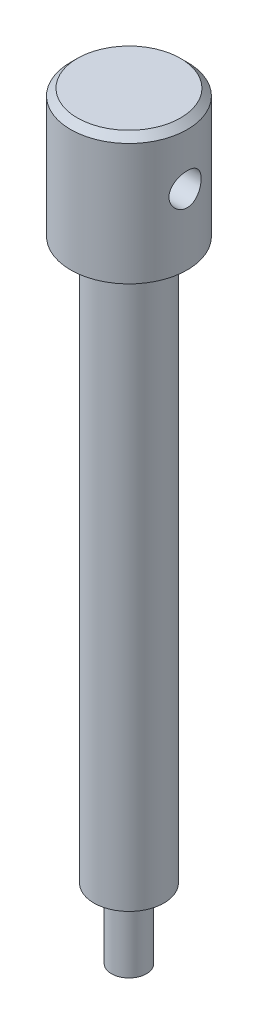
ISO-10303-21;
HEADER;
FILE_DESCRIPTION(('STEP AP214'),'2;1');
FILE_NAME('part.step','',(''),(''),'','','');
FILE_SCHEMA(('AUTOMOTIVE_DESIGN { 1 0 10303 214 1 1 1 1 }'));
ENDSEC;
DATA;
#1=APPLICATION_CONTEXT('core data for automotive mechanical design processes');
#2=APPLICATION_PROTOCOL_DEFINITION('international standard','automotive_design',2000,#1);
#3=PRODUCT_CONTEXT('',#1,'mechanical');
#4=PRODUCT('Part','Part','',(#3));
#5=PRODUCT_RELATED_PRODUCT_CATEGORY('part','',(#4));
#6=PRODUCT_DEFINITION_FORMATION('','',#4);
#7=PRODUCT_DEFINITION_CONTEXT('part definition',#1,'design');
#8=PRODUCT_DEFINITION('design','',#6,#7);
#9=PRODUCT_DEFINITION_SHAPE('','',#8);
#10=(LENGTH_UNIT() NAMED_UNIT(*) SI_UNIT(.MILLI.,.METRE.));
#11=(NAMED_UNIT(*) PLANE_ANGLE_UNIT() SI_UNIT($,.RADIAN.));
#12=(NAMED_UNIT(*) SI_UNIT($,.STERADIAN.) SOLID_ANGLE_UNIT());
#13=UNCERTAINTY_MEASURE_WITH_UNIT(LENGTH_MEASURE(1.E-05),#10,'distance_accuracy_value','');
#14=(GEOMETRIC_REPRESENTATION_CONTEXT(3) GLOBAL_UNCERTAINTY_ASSIGNED_CONTEXT((#13)) GLOBAL_UNIT_ASSIGNED_CONTEXT((#10,
#11,#12)) REPRESENTATION_CONTEXT('',''));
#15=CARTESIAN_POINT('',(0.,0.,0.));
#16=DIRECTION('',(0.,0.,1.));
#17=DIRECTION('',(1.,0.,0.));
#18=AXIS2_PLACEMENT_3D('',#15,#16,#17);
#19=CARTESIAN_POINT('',(0.,12.,0.));
#20=DIRECTION('',(0.,-1.,0.));
#21=DIRECTION('',(0.,0.,-1.));
#22=AXIS2_PLACEMENT_3D('',#19,#20,#21);
#23=CYLINDRICAL_SURFACE('',#22,3.);
#24=CARTESIAN_POINT('',(0.,12.,0.));
#25=DIRECTION('',(0.,1.,0.));
#26=DIRECTION('',(0.,0.,1.));
#27=AXIS2_PLACEMENT_3D('',#24,#25,#26);
#28=CIRCLE('',#27,3.);
#29=CARTESIAN_POINT('',(0.,12.,3.));
#30=VERTEX_POINT('',#29);
#31=EDGE_CURVE('E52',#30,#30,#28,.T.);
#32=ORIENTED_EDGE('',*,*,#31,.F.);
#33=EDGE_LOOP('',(#32));
#34=FACE_BOUND('',#33,.T.);
#35=CARTESIAN_POINT('',(0.,0.,0.));
#36=DIRECTION('',(0.,1.,0.));
#37=DIRECTION('',(0.,0.,1.));
#38=AXIS2_PLACEMENT_3D('',#35,#36,#37);
#39=CIRCLE('',#38,3.);
#40=CARTESIAN_POINT('',(0.,0.,3.));
#41=VERTEX_POINT('',#40);
#42=EDGE_CURVE('E60',#41,#41,#39,.T.);
#43=ORIENTED_EDGE('',*,*,#42,.T.);
#44=EDGE_LOOP('',(#43));
#45=FACE_BOUND('',#44,.T.);
#46=ADVANCED_FACE('F41',(#34,#45),#23,.T.);
#47=CARTESIAN_POINT('',(0.,0.,0.));
#48=DIRECTION('',(0.,1.,0.));
#49=DIRECTION('',(0.,0.,1.));
#50=AXIS2_PLACEMENT_3D('',#47,#48,#49);
#51=PLANE('',#50);
#52=ORIENTED_EDGE('',*,*,#42,.F.);
#53=EDGE_LOOP('',(#52));
#54=FACE_BOUND('',#53,.T.);
#55=ADVANCED_FACE('F92',(#54),#51,.F.);
#56=CARTESIAN_POINT('',(0.,108.,0.));
#57=DIRECTION('',(0.,-1.,0.));
#58=DIRECTION('',(0.,0.,-1.));
#59=AXIS2_PLACEMENT_3D('',#56,#57,#58);
#60=CYLINDRICAL_SURFACE('',#59,6.);
#61=CARTESIAN_POINT('',(0.,108.,0.));
#62=DIRECTION('',(0.,1.,0.));
#63=DIRECTION('',(0.,0.,1.));
#64=AXIS2_PLACEMENT_3D('',#61,#62,#63);
#65=CIRCLE('',#64,6.);
#66=CARTESIAN_POINT('',(0.,108.,6.));
#67=VERTEX_POINT('',#66);
#68=EDGE_CURVE('E116',#67,#67,#65,.T.);
#69=ORIENTED_EDGE('',*,*,#68,.F.);
#70=EDGE_LOOP('',(#69));
#71=FACE_BOUND('',#70,.T.);
#72=CARTESIAN_POINT('',(0.,12.,0.));
#73=DIRECTION('',(0.,1.,0.));
#74=DIRECTION('',(0.,0.,1.));
#75=AXIS2_PLACEMENT_3D('',#72,#73,#74);
#76=CIRCLE('',#75,6.);
#77=CARTESIAN_POINT('',(0.,12.,6.));
#78=VERTEX_POINT('',#77);
#79=EDGE_CURVE('E118',#78,#78,#76,.T.);
#80=ORIENTED_EDGE('',*,*,#79,.T.);
#81=EDGE_LOOP('',(#80));
#82=FACE_BOUND('',#81,.T.);
#83=ADVANCED_FACE('F99',(#71,#82),#60,.T.);
#84=CARTESIAN_POINT('',(0.,12.,0.));
#85=DIRECTION('',(0.,1.,0.));
#86=DIRECTION('',(0.,0.,1.));
#87=AXIS2_PLACEMENT_3D('',#84,#85,#86);
#88=PLANE('',#87);
#89=ORIENTED_EDGE('',*,*,#31,.T.);
#90=EDGE_LOOP('',(#89));
#91=FACE_BOUND('',#90,.T.);
#92=ORIENTED_EDGE('',*,*,#79,.F.);
#93=EDGE_LOOP('',(#92));
#94=FACE_BOUND('',#93,.T.);
#95=ADVANCED_FACE('F110',(#91,#94),#88,.F.);
#96=CARTESIAN_POINT('',(0.,130.,0.));
#97=DIRECTION('',(0.,-1.,0.));
#98=DIRECTION('',(0.,0.,-1.));
#99=AXIS2_PLACEMENT_3D('',#96,#97,#98);
#100=CYLINDRICAL_SURFACE('',#99,10.);
#101=CARTESIAN_POINT('',(0.,128.85,0.));
#102=DIRECTION('',(0.,1.,0.));
#103=DIRECTION('',(0.,0.,1.));
#104=AXIS2_PLACEMENT_3D('',#101,#102,#103);
#105=CIRCLE('',#104,10.);
#106=CARTESIAN_POINT('',(0.,128.85,10.));
#107=VERTEX_POINT('',#106);
#108=EDGE_CURVE('E10',#107,#107,#105,.F.);
#109=ORIENTED_EDGE('',*,*,#108,.T.);
#110=EDGE_LOOP('',(#109));
#111=FACE_BOUND('',#110,.T.);
#112=CARTESIAN_POINT('',(-9.61444226151471,120.,-2.75));
#113=CARTESIAN_POINT('',(-9.61444469239416,120.151300744405,-2.74999672907596));
#114=CARTESIAN_POINT('',(-9.61805280816712,120.30263538436,-2.73747096923585));
#115=CARTESIAN_POINT('',(-9.63204886497316,120.600921179537,-2.68780188601347));
#116=CARTESIAN_POINT('',(-9.64243992812534,120.747870283555,-2.65064722608637));
#117=CARTESIAN_POINT('',(-9.66873799316869,121.033026311981,-2.55304447855365));
#118=CARTESIAN_POINT('',(-9.68463690010815,121.171245716006,-2.49263056096248));
#119=CARTESIAN_POINT('',(-9.72014878041224,121.435612030258,-2.35033265308946));
#120=CARTESIAN_POINT('',(-9.73976210867894,121.561757785148,-2.26844661092129));
#121=CARTESIAN_POINT('',(-9.78107754816646,121.801750770529,-2.0831994086483));
#122=CARTESIAN_POINT('',(-9.80281854438383,121.915229352047,-1.979369224386));
#123=CARTESIAN_POINT('',(-9.84560488395749,122.123402002932,-1.75418896845015));
#124=CARTESIAN_POINT('',(-9.86665015106763,122.218094019097,-1.6328369843032));
#125=CARTESIAN_POINT('',(-9.9061095943824,122.387558006288,-1.37348569653624));
#126=CARTESIAN_POINT('',(-9.9244725631045,122.461961227299,-1.23523697719301));
#127=CARTESIAN_POINT('',(-9.95605089602316,122.586326897958,-0.947602230959203));
#128=CARTESIAN_POINT('',(-9.96926718549175,122.636293741203,-0.798218211736089));
#129=CARTESIAN_POINT('',(-9.98878804836854,122.709168741138,-0.496403517981859));
#130=CARTESIAN_POINT('',(-9.99525267253508,122.732704526695,-0.344134922828677));
#131=CARTESIAN_POINT('',(-10.0011023830534,122.754026331133,-0.0376824378667688));
#132=CARTESIAN_POINT('',(-10.0004887265994,122.751816922694,0.116501106962677));
#133=CARTESIAN_POINT('',(-9.99236730085294,122.722148089349,0.418030007781093));
#134=CARTESIAN_POINT('',(-9.98504478048099,122.695367120028,0.565447876976582));
#135=CARTESIAN_POINT('',(-9.96454853894465,122.618414359012,0.853610400052433));
#136=CARTESIAN_POINT('',(-9.95137447394198,122.568241192776,0.994354661251917));
#137=CARTESIAN_POINT('',(-9.92038512273078,122.445423090756,1.26687794984864));
#138=CARTESIAN_POINT('',(-9.90252308604197,122.372550333144,1.39854876994441));
#139=CARTESIAN_POINT('',(-9.86407534097692,122.206577680589,1.64802088098144));
#140=CARTESIAN_POINT('',(-9.84348907323179,122.113473629008,1.76581931407912));
#141=CARTESIAN_POINT('',(-9.80102554909703,121.906098981135,1.98825308222214));
#142=CARTESIAN_POINT('',(-9.77912808432924,121.791237424021,2.09233427623928));
#143=CARTESIAN_POINT('',(-9.73711103860844,121.545465963472,2.27989747699747));
#144=CARTESIAN_POINT('',(-9.71699158083097,121.414554949671,2.36337805730045));
#145=CARTESIAN_POINT('',(-9.68072344726396,121.139138205135,2.50782839605253));
#146=CARTESIAN_POINT('',(-9.66460320549397,120.994544687894,2.56863842235454));
#147=CARTESIAN_POINT('',(-9.63850727059708,120.696630641825,2.66490015227663));
#148=CARTESIAN_POINT('',(-9.62852994166518,120.543312448195,2.70035860720866));
#149=CARTESIAN_POINT('',(-9.61620058867586,120.237505982008,2.74393630541318));
#150=CARTESIAN_POINT('',(-9.61361703809613,120.085145253441,2.75288596156733));
#151=CARTESIAN_POINT('',(-9.61573265646036,119.781102449334,2.74548746374689));
#152=CARTESIAN_POINT('',(-9.62043099390854,119.629420298293,2.72914219811978));
#153=CARTESIAN_POINT('',(-9.63635647166543,119.334301868875,2.67235183466837));
#154=CARTESIAN_POINT('',(-9.64744599186171,119.190759761204,2.63241430491429));
#155=CARTESIAN_POINT('',(-9.67476791667406,118.912413861308,2.53014801391641));
#156=CARTESIAN_POINT('',(-9.69100102383443,118.777611265813,2.46781619376014));
#157=CARTESIAN_POINT('',(-9.7272499264732,118.517119843033,2.32087173142269));
#158=CARTESIAN_POINT('',(-9.74734468881971,118.391714736464,2.23577607047318));
#159=CARTESIAN_POINT('',(-9.78887094072755,118.156659395667,2.04631207337349));
#160=CARTESIAN_POINT('',(-9.81030269752423,118.047012325681,1.94193987604753));
#161=CARTESIAN_POINT('',(-9.85289165657554,117.843094408271,1.71302917650185));
#162=CARTESIAN_POINT('',(-9.87401979289675,117.749405024988,1.58796617241509));
#163=CARTESIAN_POINT('',(-9.91294281659086,117.584344949263,1.32340991078638));
#164=CARTESIAN_POINT('',(-9.93073788102544,117.512973071119,1.18391742038877));
#165=CARTESIAN_POINT('',(-9.96087510629648,117.395242644478,0.895441697256458));
#166=CARTESIAN_POINT('',(-9.97325824848057,117.348695498441,0.74653992401912));
#167=CARTESIAN_POINT('',(-9.99135709268039,117.281400805053,0.442633863292109));
#168=CARTESIAN_POINT('',(-9.99707437357267,117.260647148178,0.287631029895586));
#169=CARTESIAN_POINT('',(-10.0011175281841,117.245931349314,-0.0186597955150437));
#170=CARTESIAN_POINT('',(-9.99967803199252,117.251118779561,-0.169904391351267));
#171=CARTESIAN_POINT('',(-9.99010535858289,117.286149303016,-0.469282591094472));
#172=CARTESIAN_POINT('',(-9.98197246168843,117.315991363675,-0.617416325019769));
#173=CARTESIAN_POINT('',(-9.95997850262577,117.398991268148,-0.905276243065433));
#174=CARTESIAN_POINT('',(-9.94616225051978,117.451966913484,-1.04505861353937));
#175=CARTESIAN_POINT('',(-9.91424169259157,117.579568054387,-1.31382994403439));
#176=CARTESIAN_POINT('',(-9.8961367570928,117.654196729475,-1.44281731533626));
#177=CARTESIAN_POINT('',(-9.85693540766064,117.825420059975,-1.69025672012208));
#178=CARTESIAN_POINT('',(-9.83576940123647,117.922571482097,-1.80831241023403));
#179=CARTESIAN_POINT('',(-9.79309788223025,118.135039544075,-2.02673246336397));
#180=CARTESIAN_POINT('',(-9.77159227993218,118.250361058954,-2.12709206317733));
#181=CARTESIAN_POINT('',(-9.73008379901748,118.499196341971,-2.30964502111673));
#182=CARTESIAN_POINT('',(-9.71012886862592,118.633077771907,-2.39134915894197));
#183=CARTESIAN_POINT('',(-9.67467721353604,118.913209343242,-2.53097682703811));
#184=CARTESIAN_POINT('',(-9.65917775226623,119.05945182068,-2.58891496388418));
#185=CARTESIAN_POINT('',(-9.63639905608115,119.337493887027,-2.67233659578139));
#186=CARTESIAN_POINT('',(-9.62823443148593,119.468160413371,-2.70138929663034));
#187=CARTESIAN_POINT('',(-9.61725531174262,119.732542733901,-2.74022117661163));
#188=CARTESIAN_POINT('',(-9.61444011274552,119.866258124591,-2.75000289132428));
#189=CARTESIAN_POINT('',(-9.61444226151471,120.,-2.75));
#190=B_SPLINE_CURVE_WITH_KNOTS('',3,(#112,#113,#114,#115,#116,#117,#118,#119,#120,#121,#122,
#123,#124,#125,#126,#127,#128,#129,#130,#131,#132,#133,#134,#135,#136,#137,#138,#139,#140,#141,
#142,#143,#144,#145,#146,#147,#148,#149,#150,#151,#152,#153,#154,#155,#156,#157,#158,#159,#160,
#161,#162,#163,#164,#165,#166,#167,#168,#169,#170,#171,#172,#173,#174,#175,#176,#177,#178,#179,
#180,#181,#182,#183,#184,#185,#186,#187,#188,#189),.UNSPECIFIED.,.T.,.F.,(4,2,2,2,2,2,2,2,2,2,2,
2,2,2,2,2,2,2,2,2,2,2,2,2,2,2,2,2,2,2,2,2,2,2,2,2,2,2,4),(0.,0.453410085173355,0.90702901752605,
1.35998406880197,1.81298242045979,2.27687307477619,2.74081440026421,3.21269770308402,
3.68449613132672,4.14483737202103,4.60509685140574,5.05301832403501,5.50096612012863,
5.95356300267944,6.40625296198359,6.87369697745072,7.34117335083543,7.81188386419097,
8.2824689770985,8.73814794986568,9.19377489392485,9.63993914074728,10.0861643538495,
10.5427340102772,10.9993952190132,11.4702011934689,11.9409821503539,12.4081336340194,
12.8751744456454,13.3270066073928,13.7788198471023,14.2271370679707,14.6755201528778,
15.1364637156438,15.5975311604638,16.069572333148,16.5413229532469,16.9421662910629,
17.3429568843874),.UNSPECIFIED.);
#191=CARTESIAN_POINT('',(-9.61444226151471,120.,-2.75));
#192=VERTEX_POINT('',#191);
#193=EDGE_CURVE('E58',#192,#192,#190,.T.);
#194=ORIENTED_EDGE('',*,*,#193,.T.);
#195=EDGE_LOOP('',(#194));
#196=FACE_BOUND('',#195,.T.);
#197=CARTESIAN_POINT('',(9.61444226151471,120.,-2.75));
#198=CARTESIAN_POINT('',(9.61444469239416,119.848699255595,-2.74999672907596));
#199=CARTESIAN_POINT('',(9.61805280816712,119.69736461564,-2.73747096923585));
#200=CARTESIAN_POINT('',(9.63204886497316,119.399078820463,-2.68780188601347));
#201=CARTESIAN_POINT('',(9.64243992812534,119.252129716445,-2.65064722608637));
#202=CARTESIAN_POINT('',(9.66873799316869,118.96697368802,-2.55304447855365));
#203=CARTESIAN_POINT('',(9.68463690010815,118.828754283994,-2.49263056096248));
#204=CARTESIAN_POINT('',(9.72014878041224,118.564387969742,-2.35033265308946));
#205=CARTESIAN_POINT('',(9.73976210867894,118.438242214852,-2.26844661092129));
#206=CARTESIAN_POINT('',(9.78107754816646,118.198249229471,-2.0831994086483));
#207=CARTESIAN_POINT('',(9.80281854438383,118.084770647953,-1.979369224386));
#208=CARTESIAN_POINT('',(9.84560488395749,117.876597997068,-1.75418896845015));
#209=CARTESIAN_POINT('',(9.86665015106763,117.781905980904,-1.6328369843032));
#210=CARTESIAN_POINT('',(9.9061095943824,117.612441993712,-1.37348569653624));
#211=CARTESIAN_POINT('',(9.9244725631045,117.538038772702,-1.23523697719301));
#212=CARTESIAN_POINT('',(9.95605089602316,117.413673102042,-0.947602230959201));
#213=CARTESIAN_POINT('',(9.96926718549175,117.363706258797,-0.798218211736087));
#214=CARTESIAN_POINT('',(9.98878804836854,117.290831258862,-0.496403517981858));
#215=CARTESIAN_POINT('',(9.99525267253508,117.267295473306,-0.344134922828676));
#216=CARTESIAN_POINT('',(10.0011023830534,117.245973668867,-0.0376824378667689));
#217=CARTESIAN_POINT('',(10.0004887265994,117.248183077306,0.116501106962677));
#218=CARTESIAN_POINT('',(9.99236730085294,117.277851910652,0.418030007781092));
#219=CARTESIAN_POINT('',(9.98504478048099,117.304632879972,0.56544787697658));
#220=CARTESIAN_POINT('',(9.96454853894465,117.381585640989,0.853610400052431));
#221=CARTESIAN_POINT('',(9.95137447394198,117.431758807224,0.994354661251916));
#222=CARTESIAN_POINT('',(9.92038512273078,117.554576909245,1.26687794984864));
#223=CARTESIAN_POINT('',(9.90252308604197,117.627449666857,1.39854876994441));
#224=CARTESIAN_POINT('',(9.86407534097692,117.793422319411,1.64802088098144));
#225=CARTESIAN_POINT('',(9.84348907323179,117.886526370992,1.76581931407912));
#226=CARTESIAN_POINT('',(9.80102554909703,118.093901018866,1.98825308222214));
#227=CARTESIAN_POINT('',(9.77912808432924,118.208762575979,2.09233427623928));
#228=CARTESIAN_POINT('',(9.73711103860844,118.454534036528,2.27989747699747));
#229=CARTESIAN_POINT('',(9.71699158083097,118.585445050329,2.36337805730045));
#230=CARTESIAN_POINT('',(9.68072344726396,118.860861794865,2.50782839605254));
#231=CARTESIAN_POINT('',(9.66460320549397,119.005455312106,2.56863842235454));
#232=CARTESIAN_POINT('',(9.63850727059708,119.303369358175,2.66490015227663));
#233=CARTESIAN_POINT('',(9.62852994166518,119.456687551805,2.70035860720866));
#234=CARTESIAN_POINT('',(9.61620058867586,119.762494017992,2.74393630541318));
#235=CARTESIAN_POINT('',(9.61361703809613,119.91485474656,2.75288596156733));
#236=CARTESIAN_POINT('',(9.61573265646036,120.218897550667,2.74548746374689));
#237=CARTESIAN_POINT('',(9.62043099390854,120.370579701707,2.72914219811978));
#238=CARTESIAN_POINT('',(9.63635647166543,120.665698131126,2.67235183466837));
#239=CARTESIAN_POINT('',(9.64744599186171,120.809240238797,2.63241430491429));
#240=CARTESIAN_POINT('',(9.67476791667406,121.087586138693,2.53014801391641));
#241=CARTESIAN_POINT('',(9.69100102383443,121.222388734187,2.46781619376014));
#242=CARTESIAN_POINT('',(9.7272499264732,121.482880156967,2.32087173142269));
#243=CARTESIAN_POINT('',(9.74734468881971,121.608285263536,2.23577607047319));
#244=CARTESIAN_POINT('',(9.78887094072755,121.843340604333,2.0463120733735));
#245=CARTESIAN_POINT('',(9.81030269752423,121.952987674319,1.94193987604754));
#246=CARTESIAN_POINT('',(9.85289165657554,122.156905591729,1.71302917650185));
#247=CARTESIAN_POINT('',(9.87401979289675,122.250594975012,1.58796617241509));
#248=CARTESIAN_POINT('',(9.91294281659086,122.415655050738,1.32340991078638));
#249=CARTESIAN_POINT('',(9.93073788102544,122.487026928881,1.18391742038877));
#250=CARTESIAN_POINT('',(9.96087510629648,122.604757355522,0.895441697256457));
#251=CARTESIAN_POINT('',(9.97325824848057,122.65130450156,0.746539924019118));
#252=CARTESIAN_POINT('',(9.99135709268039,122.718599194947,0.442633863292107));
#253=CARTESIAN_POINT('',(9.99707437357267,122.739352851822,0.287631029895585));
#254=CARTESIAN_POINT('',(10.0011175281841,122.754068650686,-0.0186597955150453));
#255=CARTESIAN_POINT('',(9.99967803199252,122.748881220439,-0.169904391351271));
#256=CARTESIAN_POINT('',(9.99010535858289,122.713850696984,-0.469282591094475));
#257=CARTESIAN_POINT('',(9.98197246168843,122.684008636325,-0.61741632501977));
#258=CARTESIAN_POINT('',(9.95997850262577,122.601008731853,-0.905276243065436));
#259=CARTESIAN_POINT('',(9.94616225051977,122.548033086516,-1.04505861353938));
#260=CARTESIAN_POINT('',(9.91424169259157,122.420431945613,-1.3138299440344));
#261=CARTESIAN_POINT('',(9.8961367570928,122.345803270525,-1.44281731533626));
#262=CARTESIAN_POINT('',(9.85693540766064,122.174579940025,-1.69025672012208));
#263=CARTESIAN_POINT('',(9.83576940123647,122.077428517903,-1.80831241023403));
#264=CARTESIAN_POINT('',(9.79309788223025,121.864960455925,-2.02673246336397));
#265=CARTESIAN_POINT('',(9.77159227993218,121.749638941046,-2.12709206317733));
#266=CARTESIAN_POINT('',(9.73008379901748,121.50080365803,-2.30964502111673));
#267=CARTESIAN_POINT('',(9.71012886862592,121.366922228093,-2.39134915894197));
#268=CARTESIAN_POINT('',(9.67467721353604,121.086790656758,-2.53097682703811));
#269=CARTESIAN_POINT('',(9.65917775226623,120.94054817932,-2.58891496388418));
#270=CARTESIAN_POINT('',(9.63639905608115,120.662506112973,-2.67233659578139));
#271=CARTESIAN_POINT('',(9.62823443148593,120.531839586629,-2.70138929663034));
#272=CARTESIAN_POINT('',(9.61725531174262,120.267457266099,-2.74022117661164));
#273=CARTESIAN_POINT('',(9.61444011274552,120.133741875409,-2.75000289132428));
#274=CARTESIAN_POINT('',(9.61444226151471,120.,-2.75));
#275=B_SPLINE_CURVE_WITH_KNOTS('',3,(#197,#198,#199,#200,#201,#202,#203,#204,#205,#206,#207,
#208,#209,#210,#211,#212,#213,#214,#215,#216,#217,#218,#219,#220,#221,#222,#223,#224,#225,#226,
#227,#228,#229,#230,#231,#232,#233,#234,#235,#236,#237,#238,#239,#240,#241,#242,#243,#244,#245,
#246,#247,#248,#249,#250,#251,#252,#253,#254,#255,#256,#257,#258,#259,#260,#261,#262,#263,#264,
#265,#266,#267,#268,#269,#270,#271,#272,#273,#274),.UNSPECIFIED.,.T.,.F.,(4,2,2,2,2,2,2,2,2,2,2,
2,2,2,2,2,2,2,2,2,2,2,2,2,2,2,2,2,2,2,2,2,2,2,2,2,2,2,4),(0.,0.453410085173355,0.90702901752605,
1.35998406880197,1.81298242045979,2.27687307477619,2.74081440026421,3.21269770308403,
3.68449613132672,4.14483737202104,4.60509685140575,5.05301832403501,5.50096612012864,
5.95356300267944,6.40625296198359,6.87369697745072,7.34117335083543,7.81188386419098,
8.2824689770985,8.7381479498657,9.19377489392485,9.63993914074728,10.0861643538495,
10.5427340102771,10.9993952190132,11.4702011934689,11.9409821503539,12.4081336340195,
12.8751744456454,13.3270066073928,13.7788198471023,14.2271370679707,14.6755201528778,
15.1364637156438,15.5975311604638,16.069572333148,16.5413229532469,16.942166291063,
17.3429568843874),.UNSPECIFIED.);
#276=CARTESIAN_POINT('',(9.61444226151471,120.,-2.75));
#277=VERTEX_POINT('',#276);
#278=EDGE_CURVE('E68',#277,#277,#275,.T.);
#279=ORIENTED_EDGE('',*,*,#278,.T.);
#280=EDGE_LOOP('',(#279));
#281=FACE_BOUND('',#280,.T.);
#282=CARTESIAN_POINT('',(0.,108.,0.));
#283=DIRECTION('',(0.,1.,0.));
#284=DIRECTION('',(0.,0.,1.));
#285=AXIS2_PLACEMENT_3D('',#282,#283,#284);
#286=CIRCLE('',#285,10.);
#287=CARTESIAN_POINT('',(0.,108.,10.));
#288=VERTEX_POINT('',#287);
#289=EDGE_CURVE('E67',#288,#288,#286,.T.);
#290=ORIENTED_EDGE('',*,*,#289,.T.);
#291=EDGE_LOOP('',(#290));
#292=FACE_BOUND('',#291,.T.);
#293=ADVANCED_FACE('F74',(#111,#196,#281,#292),#100,.T.);
#294=CARTESIAN_POINT('',(0.,130.,0.));
#295=DIRECTION('',(0.,1.,0.));
#296=DIRECTION('',(0.,0.,1.));
#297=AXIS2_PLACEMENT_3D('',#294,#295,#296);
#298=PLANE('',#297);
#299=CARTESIAN_POINT('',(0.,130.,0.));
#300=DIRECTION('',(0.,1.,0.));
#301=DIRECTION('',(0.,0.,1.));
#302=AXIS2_PLACEMENT_3D('',#299,#300,#301);
#303=CIRCLE('',#302,8.84999999999996);
#304=CARTESIAN_POINT('',(0.,130.,8.84999999999996));
#305=VERTEX_POINT('',#304);
#306=EDGE_CURVE('E47',#305,#305,#303,.T.);
#307=ORIENTED_EDGE('',*,*,#306,.T.);
#308=EDGE_LOOP('',(#307));
#309=FACE_BOUND('',#308,.T.);
#310=ADVANCED_FACE('F83',(#309),#298,.T.);
#311=CARTESIAN_POINT('',(0.,108.,0.));
#312=DIRECTION('',(0.,1.,0.));
#313=DIRECTION('',(0.,0.,1.));
#314=AXIS2_PLACEMENT_3D('',#311,#312,#313);
#315=PLANE('',#314);
#316=ORIENTED_EDGE('',*,*,#68,.T.);
#317=EDGE_LOOP('',(#316));
#318=FACE_BOUND('',#317,.T.);
#319=ORIENTED_EDGE('',*,*,#289,.F.);
#320=EDGE_LOOP('',(#319));
#321=FACE_BOUND('',#320,.T.);
#322=ADVANCED_FACE('F85',(#318,#321),#315,.F.);
#323=CARTESIAN_POINT('',(-11.,120.,0.));
#324=DIRECTION('',(1.,0.,0.));
#325=DIRECTION('',(0.,0.,-1.));
#326=AXIS2_PLACEMENT_3D('',#323,#324,#325);
#327=CYLINDRICAL_SURFACE('',#326,2.75);
#328=ORIENTED_EDGE('',*,*,#278,.F.);
#329=EDGE_LOOP('',(#328));
#330=FACE_BOUND('',#329,.T.);
#331=ORIENTED_EDGE('',*,*,#193,.F.);
#332=EDGE_LOOP('',(#331));
#333=FACE_BOUND('',#332,.T.);
#334=ADVANCED_FACE('F76',(#330,#333),#327,.F.);
#335=CARTESIAN_POINT('',(0.,130.,0.));
#336=DIRECTION('',(0.,-1.,0.));
#337=DIRECTION('',(0.,0.,-1.));
#338=AXIS2_PLACEMENT_3D('',#335,#336,#337);
#339=CONICAL_SURFACE('',#338,8.84999999999996,0.785398163397439);
#340=ORIENTED_EDGE('',*,*,#108,.F.);
#341=EDGE_LOOP('',(#340));
#342=FACE_BOUND('',#341,.T.);
#343=ORIENTED_EDGE('',*,*,#306,.F.);
#344=EDGE_LOOP('',(#343));
#345=FACE_BOUND('',#344,.T.);
#346=ADVANCED_FACE('F42',(#342,#345),#339,.T.);
#347=CLOSED_SHELL('',(#46,#55,#83,#95,#293,#310,#322,#334,#346));
#348=MANIFOLD_SOLID_BREP('B2',#347);
#349=ADVANCED_BREP_SHAPE_REPRESENTATION('',(#18,#348),#14);
#350=SHAPE_DEFINITION_REPRESENTATION(#9,#349);
ENDSEC;
END-ISO-10303-21;
